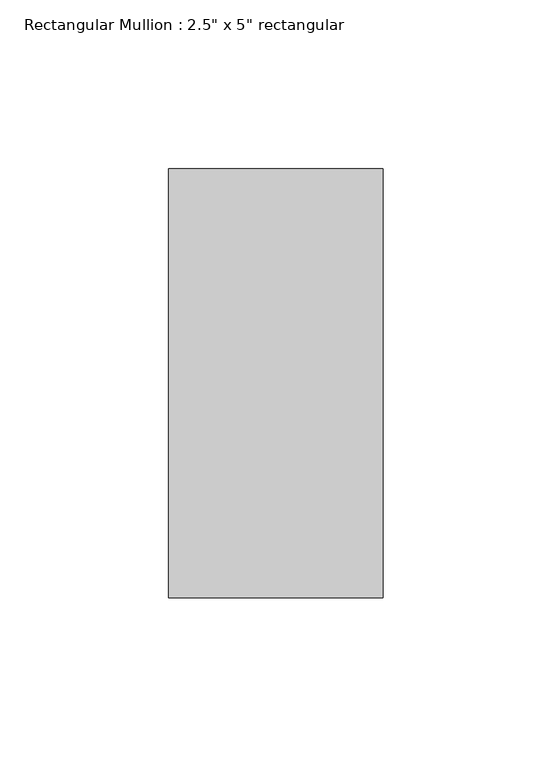
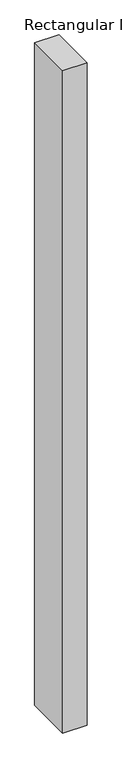
"""IFC4 building model written with IfcOpenShell, lengths in millimetres: member geometry."""

from ifc_helpers import new_model, si_unit, frame, origin, place, context, project, spatial, polyline, outline, extrude, source, transform, mapped, element, save


def member_2fae0574(model_context):
    return source(origin(), model_context, "Body", "SweptSolid", [
        extrude(outline(polyline([(0.0, 63.5), (0.0, -63.5), (-63.5, -63.5), (-63.5, 63.5), (0.0, 63.5)])), frame((0.0, 0.0, -1828.8), z_axis=(0.0, 0.0, 1.0), x_axis=(1.0, 0.0, 0.0)), (0.0, 0.0, 1.0), 1828.8),
    ])


if __name__ == "__main__":
    model = new_model("IFC4")
    model_context = context("Model", 3, world=origin())
    ifc_project = project(units=[si_unit("LENGTHUNIT", "METRE", prefix="MILLI")], contexts=[model_context])
    site = spatial("IfcSite", under=ifc_project)
    building = spatial("IfcBuilding", under=site)
    placement = place(None, origin())
    member_shape = member_2fae0574(model_context)
    element("IfcMember", 1, ObjectType="Rectangular Mullion : 2.5\" x 5\" rectangular", at=placement, inside=building, context=model_context, shape_type="MappedRepresentation", body=[
        mapped(member_shape, transform((0.0, 0.0, 0.0), x_axis=(1.0, 0.0, 0.0), y_axis=(0.0, 1.0, 0.0), z_axis=(0.0, 0.0, 1.0))),
    ])
    save(model, "model.ifc")

# Revit data of these elements
# Type "Rectangular Mullion : 2.5\" x 5\" rectangular"
#   built-in parameter 1007304 = 0.416667 (stored number, unit not read)
#   built-in parameter 1007301 = 0.104167 (stored number, unit not read)
#   built-in parameter 1007300 = 0.104167 (stored number, unit not read)
